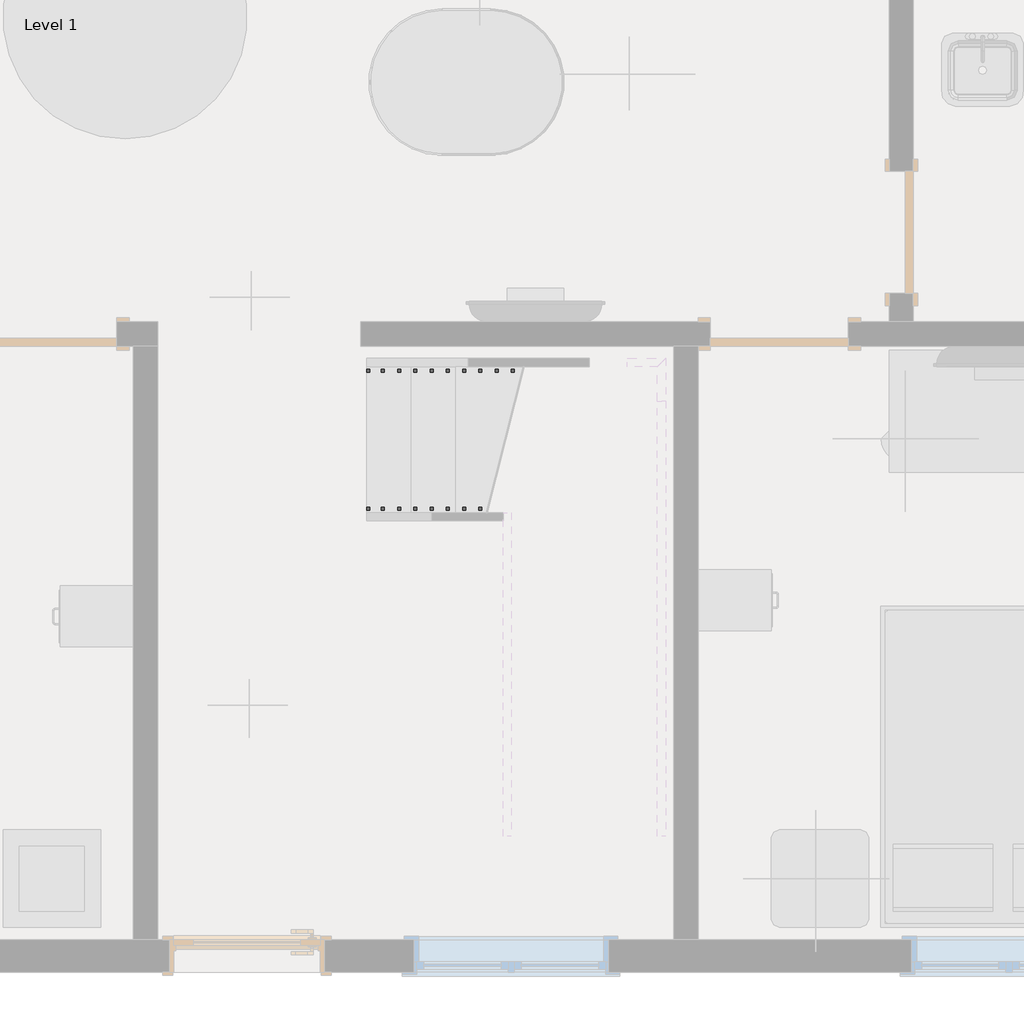
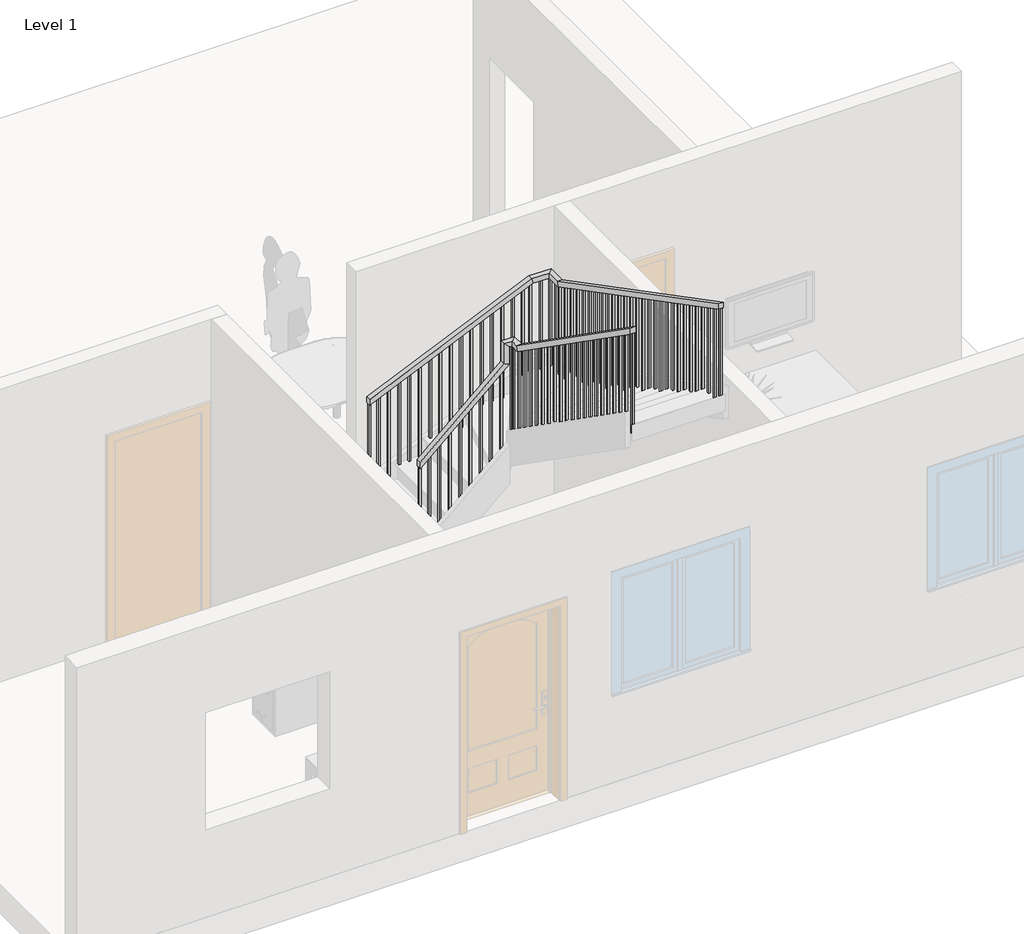
# One storey, part 2 of 3: 2 railings.
"""IFC4 building model written with IfcOpenShell, lengths in millimetres."""

from ifc_helpers import new_model, si_unit, frame, origin, place, context, project, spatial, polyline, outline, extrude, faceted_brep, element, save

model = new_model("IFC4")

# Units and contexts
model_context = context("Model", 3, world=origin())
ifc_project = project(units=[si_unit("LENGTHUNIT", "METRE", prefix="MILLI")], contexts=[model_context])

# Site, building, storey
site = spatial("IfcSite", under=ifc_project)
building = spatial("IfcBuilding", under=site)
storey = spatial("IfcBuildingStorey", under=building, Name="Level 1", Elevation=0.0)

# Railings
placement = place(None, origin())
element("IfcRailing", 1, ObjectType="Handrail - Rectangular", at=placement, inside=storey, context=model_context, shape_type="SolidModel", body=[
    faceted_brep([(-12520.2436952, 5155.3187882, 1682.9646102), (-12520.2436952, 5155.3187882, 1615.1075334), (-12520.2436952, 5104.5187882, 1615.1075334), (-12520.2436952, 5104.5187882, 1682.9646102), (-11692.5067057, 5155.3187882, 2416.0047843), (-11641.7067057, 5155.3187882, 2393.1359601), (-11641.7067057, 5104.5187882, 2393.1359601), (-11692.5067057, 5104.5187882, 2416.0047843), (-11692.5067057, 5155.3187882, 2625.457216), (-11641.7067057, 5155.3187882, 2574.657216), (-11641.7067057, 5104.5187882, 2574.657216), (-11692.5067057, 5104.5187882, 2625.457216), (-11565.5067057, 5155.3187882, 2625.457216), (-11565.5067057, 5155.3187882, 2574.657216), (-11616.3067057, 5104.5187882, 2574.657216), (-11616.3067057, 5104.5187882, 2625.457216), (-11565.5067057, 5028.3187882, 2625.457216), (-11565.5067057, 5012.2891523, 2574.657216), (-11616.3067057, 5012.2891523, 2574.657216), (-11616.3067057, 5028.3187882, 2625.457216), (-11565.5067057, 3082.9817987, 3988.8904479), (-11616.3067057, 3082.9817987, 3988.8904479), (-11616.3067057, 3082.9817987, 3926.8557166), (-11565.5067057, 3082.9817987, 3926.8557166)], [[[0, 1, 2, 3]], [[1, 0, 4, 5]], [[2, 1, 5, 6]], [[3, 2, 6, 7]], [[0, 3, 7, 4]], [[5, 4, 8, 9]], [[6, 5, 9, 10]], [[7, 6, 10, 11]], [[4, 7, 11, 8]], [[9, 8, 12, 13]], [[10, 9, 13, 14]], [[11, 10, 14, 15]], [[8, 11, 15, 12]], [[13, 12, 16, 17]], [[14, 13, 17, 18]], [[15, 14, 18, 19]], [[12, 15, 19, 16]], [[20, 21, 22, 23]], [[17, 16, 20, 23]], [[18, 17, 23, 22]], [[19, 18, 22, 21]], [[16, 19, 21, 20]]]),
    extrude(outline(polyline([(3088.3937882, 3923.0626019), (3107.4437882, 3909.7109805), (3107.4437882, 2878.6666667), (3088.3937882, 2878.6666667), (3088.3937882, 3923.0626019)])), frame((-11600.4317057, 0.0, 0.0), z_axis=(1.0, 0.0, 0.0), x_axis=(0.0, 1.0, 0.0)), (0.0, 0.0, 1.0), 19.05),
    extrude(outline(polyline([(3189.9937882, 3851.8539542), (3209.0437882, 3838.5023328), (3209.0437882, 2878.6666667), (3189.9937882, 2878.6666667), (3189.9937882, 3851.8539542)])), frame((-11600.4317057, 0.0, 0.0), z_axis=(1.0, 0.0, 0.0), x_axis=(0.0, 1.0, 0.0)), (0.0, 0.0, 1.0), 19.05),
    extrude(outline(polyline([(3291.5937882, 3780.6453065), (3310.6437882, 3767.2936851), (3310.6437882, 2878.6666667), (3291.5937882, 2878.6666667), (3291.5937882, 3780.6453065)])), frame((-11600.4317057, 0.0, 0.0), z_axis=(1.0, 0.0, 0.0), x_axis=(0.0, 1.0, 0.0)), (0.0, 0.0, 1.0), 19.05),
    extrude(outline(polyline([(3393.1937882, 3709.4366588), (3412.2437882, 3696.0850374), (3412.2437882, 2709.3333333), (3393.1937882, 2709.3333333), (3393.1937882, 3709.4366588)])), frame((-11600.4317057, 0.0, 0.0), z_axis=(1.0, 0.0, 0.0), x_axis=(0.0, 1.0, 0.0)), (0.0, 0.0, 1.0), 19.05),
    extrude(outline(polyline([(3494.7937882, 3638.2280111), (3513.8437882, 3624.8763897), (3513.8437882, 2709.3333333), (3494.7937882, 2709.3333333), (3494.7937882, 3638.2280111)])), frame((-11600.4317057, 0.0, 0.0), z_axis=(1.0, 0.0, 0.0), x_axis=(0.0, 1.0, 0.0)), (0.0, 0.0, 1.0), 19.05),
    extrude(outline(polyline([(3596.3937882, 3567.0193634), (3615.4437882, 3553.667742), (3615.4437882, 2709.3333333), (3596.3937882, 2709.3333333), (3596.3937882, 3567.0193634)])), frame((-11600.4317057, 0.0, 0.0), z_axis=(1.0, 0.0, 0.0), x_axis=(0.0, 1.0, 0.0)), (0.0, 0.0, 1.0), 19.05),
    extrude(outline(polyline([(3697.9937882, 3495.8107157), (3717.0437882, 3482.4590943), (3717.0437882, 2540.0), (3697.9937882, 2540.0), (3697.9937882, 3495.8107157)])), frame((-11600.4317057, 0.0, 0.0), z_axis=(1.0, 0.0, 0.0), x_axis=(0.0, 1.0, 0.0)), (0.0, 0.0, 1.0), 19.05),
    extrude(outline(polyline([(3799.5937882, 3424.602068), (3818.6437882, 3411.2504466), (3818.6437882, 2540.0), (3799.5937882, 2540.0), (3799.5937882, 3424.602068)])), frame((-11600.4317057, 0.0, 0.0), z_axis=(1.0, 0.0, 0.0), x_axis=(0.0, 1.0, 0.0)), (0.0, 0.0, 1.0), 19.05),
    extrude(outline(polyline([(3901.1937882, 3353.3934203), (3920.2437882, 3340.0417989), (3920.2437882, 2370.6666667), (3901.1937882, 2370.6666667), (3901.1937882, 3353.3934203)])), frame((-11600.4317057, 0.0, 0.0), z_axis=(1.0, 0.0, 0.0), x_axis=(0.0, 1.0, 0.0)), (0.0, 0.0, 1.0), 19.05),
    extrude(outline(polyline([(4002.7937882, 3282.1847726), (4021.8437882, 3268.8331511), (4021.8437882, 2370.6666667), (4002.7937882, 2370.6666667), (4002.7937882, 3282.1847726)])), frame((-11600.4317057, 0.0, 0.0), z_axis=(1.0, 0.0, 0.0), x_axis=(0.0, 1.0, 0.0)), (0.0, 0.0, 1.0), 19.05),
    extrude(outline(polyline([(4104.3937882, 3210.9761249), (4123.4437882, 3197.6245034), (4123.4437882, 2370.6666667), (4104.3937882, 2370.6666667), (4104.3937882, 3210.9761249)])), frame((-11600.4317057, 0.0, 0.0), z_axis=(1.0, 0.0, 0.0), x_axis=(0.0, 1.0, 0.0)), (0.0, 0.0, 1.0), 19.05),
    extrude(outline(polyline([(4205.9937882, 3139.7674772), (4225.0437882, 3126.4158557), (4225.0437882, 2201.3333333), (4205.9937882, 2201.3333333), (4205.9937882, 3139.7674772)])), frame((-11600.4317057, 0.0, 0.0), z_axis=(1.0, 0.0, 0.0), x_axis=(0.0, 1.0, 0.0)), (0.0, 0.0, 1.0), 19.05),
    extrude(outline(polyline([(4307.5937882, 3068.5588295), (4326.6437882, 3055.207208), (4326.6437882, 2201.3333333), (4307.5937882, 2201.3333333), (4307.5937882, 3068.5588295)])), frame((-11600.4317057, 0.0, 0.0), z_axis=(1.0, 0.0, 0.0), x_axis=(0.0, 1.0, 0.0)), (0.0, 0.0, 1.0), 19.05),
    extrude(outline(polyline([(4409.1937882, 2997.3501818), (4428.2437882, 2983.9985603), (4428.2437882, 2201.3333333), (4409.1937882, 2201.3333333), (4409.1937882, 2997.3501818)])), frame((-11600.4317057, 0.0, 0.0), z_axis=(1.0, 0.0, 0.0), x_axis=(0.0, 1.0, 0.0)), (0.0, 0.0, 1.0), 19.05),
    extrude(outline(polyline([(4510.7937882, 2926.1415341), (4529.8437882, 2912.7899126), (4529.8437882, 2032.0), (4510.7937882, 2032.0), (4510.7937882, 2926.1415341)])), frame((-11600.4317057, 0.0, 0.0), z_axis=(1.0, 0.0, 0.0), x_axis=(0.0, 1.0, 0.0)), (0.0, 0.0, 1.0), 19.05),
    extrude(outline(polyline([(4612.3937882, 2854.9328864), (4631.4437882, 2841.5812649), (4631.4437882, 2032.0), (4612.3937882, 2032.0), (4612.3937882, 2854.9328864)])), frame((-11600.4317057, 0.0, 0.0), z_axis=(1.0, 0.0, 0.0), x_axis=(0.0, 1.0, 0.0)), (0.0, 0.0, 1.0), 19.05),
    extrude(outline(polyline([(4713.9937882, 2783.7242387), (4733.0437882, 2770.3726172), (4733.0437882, 1862.6666667), (4713.9937882, 1862.6666667), (4713.9937882, 2783.7242387)])), frame((-11600.4317057, 0.0, 0.0), z_axis=(1.0, 0.0, 0.0), x_axis=(0.0, 1.0, 0.0)), (0.0, 0.0, 1.0), 19.05),
    extrude(outline(polyline([(4815.5937882, 2712.515591), (4834.6437882, 2699.1639695), (4834.6437882, 1862.6666667), (4815.5937882, 1862.6666667), (4815.5937882, 2712.515591)])), frame((-11600.4317057, 0.0, 0.0), z_axis=(1.0, 0.0, 0.0), x_axis=(0.0, 1.0, 0.0)), (0.0, 0.0, 1.0), 19.05),
    extrude(outline(polyline([(4917.1937882, 2641.3069432), (4936.2437882, 2627.9553218), (4936.2437882, 1693.3333333), (4917.1937882, 1693.3333333), (4917.1937882, 2641.3069432)])), frame((-11600.4317057, 0.0, 0.0), z_axis=(1.0, 0.0, 0.0), x_axis=(0.0, 1.0, 0.0)), (0.0, 0.0, 1.0), 19.05),
    extrude(outline(polyline([(-11600.4317057, 5037.8437882), (-11581.3817057, 5037.8437882), (-11581.3817057, 5018.7937882), (-11600.4317057, 5018.7937882), (-11600.4317057, 5037.8437882)])), frame((0.0, 0.0, 1693.3333333), z_axis=(0.0, 0.0, 1.0), x_axis=(1.0, 0.0, 0.0)), (0.0, 0.0, 1.0), 881.3238827),
    extrude(outline(polyline([(-11615.3686952, 5120.3937882), (-11615.3686952, 5139.4437882), (-11596.3186952, 5139.4437882), (-11596.3186952, 5120.3937882), (-11615.3686952, 5120.3937882)])), frame((0.0, 0.0, 1524.0), z_axis=(0.0, 0.0, 1.0), x_axis=(1.0, 0.0, 0.0)), (0.0, 0.0, 1.0), 1050.657216),
    extrude(outline(polyline([(2343.3548737, -11697.9186952), (2326.484279, -11716.9686952), (1354.6666667, -11716.9686952), (1354.6666667, -11697.9186952), (2343.3548737, -11697.9186952)])), frame((0.0, 5120.3937882, 0.0), z_axis=(0.0, 1.0, 0.0), x_axis=(0.0, 0.0, 1.0)), (0.0, 0.0, 1.0), 19.05),
    extrude(outline(polyline([(2253.3783684, -11799.5186952), (2236.5077736, -11818.5686952), (1185.3333333, -11818.5686952), (1185.3333333, -11799.5186952), (2253.3783684, -11799.5186952)])), frame((0.0, 5120.3937882, 0.0), z_axis=(0.0, 1.0, 0.0), x_axis=(0.0, 0.0, 1.0)), (0.0, 0.0, 1.0), 19.05),
    extrude(outline(polyline([(2163.401863, -11901.1186952), (2146.5312682, -11920.1686952), (1185.3333333, -11920.1686952), (1185.3333333, -11901.1186952), (2163.401863, -11901.1186952)])), frame((0.0, 5120.3937882, 0.0), z_axis=(0.0, 1.0, 0.0), x_axis=(0.0, 0.0, 1.0)), (0.0, 0.0, 1.0), 19.05),
    extrude(outline(polyline([(2073.4253576, -12002.7186952), (2056.5547629, -12021.7686952), (1016.0, -12021.7686952), (1016.0, -12002.7186952), (2073.4253576, -12002.7186952)])), frame((0.0, 5120.3937882, 0.0), z_axis=(0.0, 1.0, 0.0), x_axis=(0.0, 0.0, 1.0)), (0.0, 0.0, 1.0), 19.05),
    extrude(outline(polyline([(1983.4488522, -12104.3186952), (1966.5782575, -12123.3686952), (1016.0, -12123.3686952), (1016.0, -12104.3186952), (1983.4488522, -12104.3186952)])), frame((0.0, 5120.3937882, 0.0), z_axis=(0.0, 1.0, 0.0), x_axis=(0.0, 0.0, 1.0)), (0.0, 0.0, 1.0), 19.05),
    extrude(outline(polyline([(1893.4723469, -12205.9186952), (1876.6017521, -12224.9686952), (1016.0, -12224.9686952), (1016.0, -12205.9186952), (1893.4723469, -12205.9186952)])), frame((0.0, 5120.3937882, 0.0), z_axis=(0.0, 1.0, 0.0), x_axis=(0.0, 0.0, 1.0)), (0.0, 0.0, 1.0), 19.05),
    extrude(outline(polyline([(1803.4958415, -12307.5186952), (1786.6252467, -12326.5686952), (846.6666667, -12326.5686952), (846.6666667, -12307.5186952), (1803.4958415, -12307.5186952)])), frame((0.0, 5120.3937882, 0.0), z_axis=(0.0, 1.0, 0.0), x_axis=(0.0, 0.0, 1.0)), (0.0, 0.0, 1.0), 19.05),
    extrude(outline(polyline([(1713.5193361, -12409.1186952), (1696.6487414, -12428.1686952), (846.6666667, -12428.1686952), (846.6666667, -12409.1186952), (1713.5193361, -12409.1186952)])), frame((0.0, 5120.3937882, 0.0), z_axis=(0.0, 1.0, 0.0), x_axis=(0.0, 0.0, 1.0)), (0.0, 0.0, 1.0), 19.05),
    extrude(outline(polyline([(-11600.4317057, 5139.4437882), (-11581.3817057, 5139.4437882), (-11581.3817057, 5120.3937882), (-11600.4317057, 5120.3937882), (-11600.4317057, 5139.4437882)])), frame((0.0, 0.0, 1524.0), z_axis=(0.0, 0.0, 1.0), x_axis=(1.0, 0.0, 0.0)), (0.0, 0.0, 1.0), 1050.657216),
    extrude(outline(polyline([(3082.9817987, 3926.8557166), (3102.0317987, 3913.5040952), (3102.0317987, 2878.6666667), (3082.9817987, 2878.6666667), (3082.9817987, 3926.8557166)])), frame((-11600.4317057, 0.0, 0.0), z_axis=(1.0, 0.0, 0.0), x_axis=(0.0, 1.0, 0.0)), (0.0, 0.0, 1.0), 19.05),
    extrude(outline(polyline([(1631.9781281, -12501.1936952), (1615.1075334, -12520.2436952), (846.6666667, -12520.2436952), (846.6666667, -12501.1936952), (1631.9781281, -12501.1936952)])), frame((0.0, 5120.3937882, 0.0), z_axis=(0.0, 1.0, 0.0), x_axis=(0.0, 0.0, 1.0)), (0.0, 0.0, 1.0), 19.05),
])
element("IfcRailing", 2, ObjectType="Handrail - Rectangular", at=placement, inside=storey, context=model_context, shape_type="SolidModel", body=[
    faceted_brep([(-12520.2436952, 6018.9187882, 1807.8545254), (-12520.2436952, 6018.9187882, 1752.3830665), (-12520.2436952, 5968.1187882, 1752.3830665), (-12520.2436952, 5968.1187882, 1807.8545254), (-10922.8906609, 6018.9187882, 2508.4571941), (-10912.2398749, 6018.9187882, 2457.6571941), (-10912.2398749, 5968.1187882, 2457.6571941), (-10922.8906609, 5968.1187882, 2508.4571941), (-10701.9067057, 6018.9187882, 2508.4571941), (-10701.9067057, 6018.9187882, 2457.6571941), (-10752.7067057, 5968.1187882, 2457.6571941), (-10752.7067057, 5968.1187882, 2508.4571941), (-10701.9067057, 5828.8154443, 2508.4571941), (-10701.9067057, 5816.3790497, 2457.6571941), (-10752.7067057, 5816.3790497, 2457.6571941), (-10752.7067057, 5828.8154443, 2508.4571941), (-10701.9067057, 3082.9817987, 3938.588476), (-10752.7067057, 3082.9817987, 3938.588476), (-10752.7067057, 3082.9817987, 3881.3111437), (-10701.9067057, 3082.9817987, 3881.3111437)], [[[0, 1, 2, 3]], [[1, 0, 4, 5]], [[2, 1, 5, 6]], [[3, 2, 6, 7]], [[0, 3, 7, 4]], [[5, 4, 8, 9]], [[6, 5, 9, 10]], [[7, 6, 10, 11]], [[4, 7, 11, 8]], [[9, 8, 12, 13]], [[10, 9, 13, 14]], [[11, 10, 14, 15]], [[8, 11, 15, 12]], [[16, 17, 18, 19]], [[13, 12, 16, 19]], [[14, 13, 19, 18]], [[15, 14, 18, 17]], [[12, 15, 17, 16]]]),
    extrude(outline(polyline([(3095.1404443, 3874.9727949), (3095.1404443, 2878.6666667), (3076.0904443, 2878.6666667), (3076.0904443, 3884.8947365), (3095.1404443, 3874.9727949)])), frame((-10736.8317057, 0.0, 0.0), z_axis=(1.0, 0.0, 0.0), x_axis=(0.0, 1.0, 0.0)), (0.0, 0.0, 1.0), 19.05),
    extrude(outline(polyline([(3196.7404443, 3822.0557734), (3196.7404443, 2878.6666667), (3177.6904443, 2878.6666667), (3177.6904443, 3831.9777149), (3196.7404443, 3822.0557734)])), frame((-10736.8317057, 0.0, 0.0), z_axis=(1.0, 0.0, 0.0), x_axis=(0.0, 1.0, 0.0)), (0.0, 0.0, 1.0), 19.05),
    extrude(outline(polyline([(3298.3404443, 3769.1444302), (3298.3404443, 2878.6666667), (3279.2904443, 2878.6666667), (3279.2904443, 3779.0663717), (3298.3404443, 3769.1444302)])), frame((-10736.8317057, 0.0, 0.0), z_axis=(1.0, 0.0, 0.0), x_axis=(0.0, 1.0, 0.0)), (0.0, 0.0, 1.0), 19.05),
    extrude(outline(polyline([(3399.9404443, 3716.2217303), (3399.9404443, 2709.3333333), (3380.8904443, 2709.3333333), (3380.8904443, 3726.1436718), (3399.9404443, 3716.2217303)])), frame((-10736.8317057, 0.0, 0.0), z_axis=(1.0, 0.0, 0.0), x_axis=(0.0, 1.0, 0.0)), (0.0, 0.0, 1.0), 19.05),
    extrude(outline(polyline([(3501.5404443, 3663.3047087), (3501.5404443, 2709.3333333), (3482.4904443, 2709.3333333), (3482.4904443, 3673.2266502), (3501.5404443, 3663.3047087)])), frame((-10736.8317057, 0.0, 0.0), z_axis=(1.0, 0.0, 0.0), x_axis=(0.0, 1.0, 0.0)), (0.0, 0.0, 1.0), 19.05),
    extrude(outline(polyline([(3603.1404443, 3610.3933655), (3603.1404443, 2709.3333333), (3584.0904443, 2709.3333333), (3584.0904443, 3620.315307), (3603.1404443, 3610.3933655)])), frame((-10736.8317057, 0.0, 0.0), z_axis=(1.0, 0.0, 0.0), x_axis=(0.0, 1.0, 0.0)), (0.0, 0.0, 1.0), 19.05),
    extrude(outline(polyline([(3704.7404443, 3557.4706656), (3704.7404443, 2540.0), (3685.6904443, 2540.0), (3685.6904443, 3567.3926071), (3704.7404443, 3557.4706656)])), frame((-10736.8317057, 0.0, 0.0), z_axis=(1.0, 0.0, 0.0), x_axis=(0.0, 1.0, 0.0)), (0.0, 0.0, 1.0), 19.05),
    extrude(outline(polyline([(3806.3404443, 3504.553644), (3806.3404443, 2540.0), (3787.2904443, 2540.0), (3787.2904443, 3514.4755855), (3806.3404443, 3504.553644)])), frame((-10736.8317057, 0.0, 0.0), z_axis=(1.0, 0.0, 0.0), x_axis=(0.0, 1.0, 0.0)), (0.0, 0.0, 1.0), 19.05),
    extrude(outline(polyline([(3907.9404443, 3451.6366224), (3907.9404443, 2540.0), (3888.8904443, 2540.0), (3888.8904443, 3461.558564), (3907.9404443, 3451.6366224)])), frame((-10736.8317057, 0.0, 0.0), z_axis=(1.0, 0.0, 0.0), x_axis=(0.0, 1.0, 0.0)), (0.0, 0.0, 1.0), 19.05),
    extrude(outline(polyline([(4009.5404443, 3398.7196009), (4009.5404443, 2370.6666667), (3990.4904443, 2370.6666667), (3990.4904443, 3408.6415424), (4009.5404443, 3398.7196009)])), frame((-10736.8317057, 0.0, 0.0), z_axis=(1.0, 0.0, 0.0), x_axis=(0.0, 1.0, 0.0)), (0.0, 0.0, 1.0), 19.05),
    extrude(outline(polyline([(4111.1404443, 3345.8025793), (4111.1404443, 2370.6666667), (4092.0904443, 2370.6666667), (4092.0904443, 3355.7245208), (4111.1404443, 3345.8025793)])), frame((-10736.8317057, 0.0, 0.0), z_axis=(1.0, 0.0, 0.0), x_axis=(0.0, 1.0, 0.0)), (0.0, 0.0, 1.0), 19.05),
    extrude(outline(polyline([(4212.7404443, 3292.8912361), (4212.7404443, 2370.6666667), (4193.6904443, 2370.6666667), (4193.6904443, 3302.8131776), (4212.7404443, 3292.8912361)])), frame((-10736.8317057, 0.0, 0.0), z_axis=(1.0, 0.0, 0.0), x_axis=(0.0, 1.0, 0.0)), (0.0, 0.0, 1.0), 19.05),
    extrude(outline(polyline([(4314.3404443, 3239.9742145), (4314.3404443, 2201.3333333), (4295.2904443, 2201.3333333), (4295.2904443, 3249.8961561), (4314.3404443, 3239.9742145)])), frame((-10736.8317057, 0.0, 0.0), z_axis=(1.0, 0.0, 0.0), x_axis=(0.0, 1.0, 0.0)), (0.0, 0.0, 1.0), 19.05),
    extrude(outline(polyline([(4415.9404443, 3187.057193), (4415.9404443, 2201.3333333), (4396.8904443, 2201.3333333), (4396.8904443, 3196.9791345), (4415.9404443, 3187.057193)])), frame((-10736.8317057, 0.0, 0.0), z_axis=(1.0, 0.0, 0.0), x_axis=(0.0, 1.0, 0.0)), (0.0, 0.0, 1.0), 19.05),
    extrude(outline(polyline([(4517.5404443, 3134.1401714), (4517.5404443, 2201.3333333), (4498.4904443, 2201.3333333), (4498.4904443, 3144.062113), (4517.5404443, 3134.1401714)])), frame((-10736.8317057, 0.0, 0.0), z_axis=(1.0, 0.0, 0.0), x_axis=(0.0, 1.0, 0.0)), (0.0, 0.0, 1.0), 19.05),
    extrude(outline(polyline([(4619.1404443, 3081.2231498), (4619.1404443, 2032.0), (4600.0904443, 2032.0), (4600.0904443, 3091.1450914), (4619.1404443, 3081.2231498)])), frame((-10736.8317057, 0.0, 0.0), z_axis=(1.0, 0.0, 0.0), x_axis=(0.0, 1.0, 0.0)), (0.0, 0.0, 1.0), 19.05),
    extrude(outline(polyline([(4720.7404443, 3028.3061283), (4720.7404443, 2032.0), (4701.6904443, 2032.0), (4701.6904443, 3038.2280698), (4720.7404443, 3028.3061283)])), frame((-10736.8317057, 0.0, 0.0), z_axis=(1.0, 0.0, 0.0), x_axis=(0.0, 1.0, 0.0)), (0.0, 0.0, 1.0), 19.05),
    extrude(outline(polyline([(4822.3404443, 2975.3891067), (4822.3404443, 2032.0), (4803.2904443, 2032.0), (4803.2904443, 2985.3110483), (4822.3404443, 2975.3891067)])), frame((-10736.8317057, 0.0, 0.0), z_axis=(1.0, 0.0, 0.0), x_axis=(0.0, 1.0, 0.0)), (0.0, 0.0, 1.0), 19.05),
    extrude(outline(polyline([(4923.9404443, 2922.4720852), (4923.9404443, 1862.6666667), (4904.8904443, 1862.6666667), (4904.8904443, 2932.3940267), (4923.9404443, 2922.4720852)])), frame((-10736.8317057, 0.0, 0.0), z_axis=(1.0, 0.0, 0.0), x_axis=(0.0, 1.0, 0.0)), (0.0, 0.0, 1.0), 19.05),
    extrude(outline(polyline([(5025.5404443, 2869.5550636), (5025.5404443, 1862.6666667), (5006.4904443, 1862.6666667), (5006.4904443, 2879.4770051), (5025.5404443, 2869.5550636)])), frame((-10736.8317057, 0.0, 0.0), z_axis=(1.0, 0.0, 0.0), x_axis=(0.0, 1.0, 0.0)), (0.0, 0.0, 1.0), 19.05),
    extrude(outline(polyline([(5127.1404443, 2816.638042), (5127.1404443, 1862.6666667), (5108.0904443, 1862.6666667), (5108.0904443, 2826.5599836), (5127.1404443, 2816.638042)])), frame((-10736.8317057, 0.0, 0.0), z_axis=(1.0, 0.0, 0.0), x_axis=(0.0, 1.0, 0.0)), (0.0, 0.0, 1.0), 19.05),
    extrude(outline(polyline([(5228.7404443, 2763.7210205), (5228.7404443, 1693.3333333), (5209.6904443, 1693.3333333), (5209.6904443, 2773.642962), (5228.7404443, 2763.7210205)])), frame((-10736.8317057, 0.0, 0.0), z_axis=(1.0, 0.0, 0.0), x_axis=(0.0, 1.0, 0.0)), (0.0, 0.0, 1.0), 19.05),
    extrude(outline(polyline([(5330.3404443, 2710.8039989), (5330.3404443, 1693.3333333), (5311.2904443, 1693.3333333), (5311.2904443, 2720.7259404), (5330.3404443, 2710.8039989)])), frame((-10736.8317057, 0.0, 0.0), z_axis=(1.0, 0.0, 0.0), x_axis=(0.0, 1.0, 0.0)), (0.0, 0.0, 1.0), 19.05),
    extrude(outline(polyline([(5431.9404443, 2657.8869773), (5431.9404443, 1693.3333333), (5412.8904443, 1693.3333333), (5412.8904443, 2667.8089189), (5431.9404443, 2657.8869773)])), frame((-10736.8317057, 0.0, 0.0), z_axis=(1.0, 0.0, 0.0), x_axis=(0.0, 1.0, 0.0)), (0.0, 0.0, 1.0), 19.05),
    extrude(outline(polyline([(5533.5404443, 2604.9699558), (5533.5404443, 1693.3333333), (5514.4904443, 1693.3333333), (5514.4904443, 2614.8918973), (5533.5404443, 2604.9699558)])), frame((-10736.8317057, 0.0, 0.0), z_axis=(1.0, 0.0, 0.0), x_axis=(0.0, 1.0, 0.0)), (0.0, 0.0, 1.0), 19.05),
    extrude(outline(polyline([(5635.1404443, 2552.0529342), (5635.1404443, 1524.0), (5616.0904443, 1524.0), (5616.0904443, 2561.9748757), (5635.1404443, 2552.0529342)])), frame((-10736.8317057, 0.0, 0.0), z_axis=(1.0, 0.0, 0.0), x_axis=(0.0, 1.0, 0.0)), (0.0, 0.0, 1.0), 19.05),
    extrude(outline(polyline([(5736.7404443, 2499.1359126), (5736.7404443, 1524.0), (5717.6904443, 1524.0), (5717.6904443, 2509.0578542), (5736.7404443, 2499.1359126)])), frame((-10736.8317057, 0.0, 0.0), z_axis=(1.0, 0.0, 0.0), x_axis=(0.0, 1.0, 0.0)), (0.0, 0.0, 1.0), 19.05),
    extrude(outline(polyline([(-10717.7817057, 5901.4437882), (-10717.7817057, 5882.3937882), (-10736.8317057, 5882.3937882), (-10736.8317057, 5901.4437882), (-10717.7817057, 5901.4437882)])), frame((0.0, 0.0, 1524.0), z_axis=(0.0, 0.0, 1.0), x_axis=(1.0, 0.0, 0.0)), (0.0, 0.0, 1.0), 933.6571941),
    extrude(outline(polyline([(-10830.8156609, 6003.0437882), (-10811.7656609, 6003.0437882), (-10811.7656609, 5983.9937882), (-10830.8156609, 5983.9937882), (-10830.8156609, 6003.0437882)])), frame((0.0, 0.0, 1524.0), z_axis=(0.0, 0.0, 1.0), x_axis=(1.0, 0.0, 0.0)), (0.0, 0.0, 1.0), 933.6571941),
    extrude(outline(polyline([(2416.6352411, -11005.7686952), (1524.0, -11005.7686952), (1524.0, -10986.7186952), (2424.9906144, -10986.7186952), (2416.6352411, -11005.7686952)])), frame((0.0, 5983.9937882, 0.0), z_axis=(0.0, 1.0, 0.0), x_axis=(0.0, 0.0, 1.0)), (0.0, 0.0, 1.0), 19.05),
    extrude(outline(polyline([(2372.0732504, -11107.3686952), (1524.0, -11107.3686952), (1524.0, -11088.3186952), (2380.4286236, -11088.3186952), (2372.0732504, -11107.3686952)])), frame((0.0, 5983.9937882, 0.0), z_axis=(0.0, 1.0, 0.0), x_axis=(0.0, 0.0, 1.0)), (0.0, 0.0, 1.0), 19.05),
    extrude(outline(polyline([(2327.5112596, -11208.9686952), (1354.6666667, -11208.9686952), (1354.6666667, -11189.9186952), (2335.8666329, -11189.9186952), (2327.5112596, -11208.9686952)])), frame((0.0, 5983.9937882, 0.0), z_axis=(0.0, 1.0, 0.0), x_axis=(0.0, 0.0, 1.0)), (0.0, 0.0, 1.0), 19.05),
    extrude(outline(polyline([(2282.9492689, -11310.5686952), (1354.6666667, -11310.5686952), (1354.6666667, -11291.5186952), (2291.3046421, -11291.5186952), (2282.9492689, -11310.5686952)])), frame((0.0, 5983.9937882, 0.0), z_axis=(0.0, 1.0, 0.0), x_axis=(0.0, 0.0, 1.0)), (0.0, 0.0, 1.0), 19.05),
    extrude(outline(polyline([(2238.3872781, -11412.1686952), (1354.6666667, -11412.1686952), (1354.6666667, -11393.1186952), (2246.7426514, -11393.1186952), (2238.3872781, -11412.1686952)])), frame((0.0, 5983.9937882, 0.0), z_axis=(0.0, 1.0, 0.0), x_axis=(0.0, 0.0, 1.0)), (0.0, 0.0, 1.0), 19.05),
    extrude(outline(polyline([(2193.8252874, -11513.7686952), (1354.6666667, -11513.7686952), (1354.6666667, -11494.7186952), (2202.1806606, -11494.7186952), (2193.8252874, -11513.7686952)])), frame((0.0, 5983.9937882, 0.0), z_axis=(0.0, 1.0, 0.0), x_axis=(0.0, 0.0, 1.0)), (0.0, 0.0, 1.0), 19.05),
    extrude(outline(polyline([(2149.2632966, -11615.3686952), (1185.3333333, -11615.3686952), (1185.3333333, -11596.3186952), (2157.6186699, -11596.3186952), (2149.2632966, -11615.3686952)])), frame((0.0, 5983.9937882, 0.0), z_axis=(0.0, 1.0, 0.0), x_axis=(0.0, 0.0, 1.0)), (0.0, 0.0, 1.0), 19.05),
    extrude(outline(polyline([(2104.7013059, -11716.9686952), (1185.3333333, -11716.9686952), (1185.3333333, -11697.9186952), (2113.0566791, -11697.9186952), (2104.7013059, -11716.9686952)])), frame((0.0, 5983.9937882, 0.0), z_axis=(0.0, 1.0, 0.0), x_axis=(0.0, 0.0, 1.0)), (0.0, 0.0, 1.0), 19.05),
    extrude(outline(polyline([(2060.1393151, -11818.5686952), (1185.3333333, -11818.5686952), (1185.3333333, -11799.5186952), (2068.4946884, -11799.5186952), (2060.1393151, -11818.5686952)])), frame((0.0, 5983.9937882, 0.0), z_axis=(0.0, 1.0, 0.0), x_axis=(0.0, 0.0, 1.0)), (0.0, 0.0, 1.0), 19.05),
    extrude(outline(polyline([(2015.5773244, -11920.1686952), (1185.3333333, -11920.1686952), (1185.3333333, -11901.1186952), (2023.9326976, -11901.1186952), (2015.5773244, -11920.1686952)])), frame((0.0, 5983.9937882, 0.0), z_axis=(0.0, 1.0, 0.0), x_axis=(0.0, 0.0, 1.0)), (0.0, 0.0, 1.0), 19.05),
    extrude(outline(polyline([(1971.0153336, -12021.7686952), (1016.0, -12021.7686952), (1016.0, -12002.7186952), (1979.3707069, -12002.7186952), (1971.0153336, -12021.7686952)])), frame((0.0, 5983.9937882, 0.0), z_axis=(0.0, 1.0, 0.0), x_axis=(0.0, 0.0, 1.0)), (0.0, 0.0, 1.0), 19.05),
    extrude(outline(polyline([(1926.4533429, -12123.3686952), (1016.0, -12123.3686952), (1016.0, -12104.3186952), (1934.8087161, -12104.3186952), (1926.4533429, -12123.3686952)])), frame((0.0, 5983.9937882, 0.0), z_axis=(0.0, 1.0, 0.0), x_axis=(0.0, 0.0, 1.0)), (0.0, 0.0, 1.0), 19.05),
    extrude(outline(polyline([(1881.8913521, -12224.9686952), (1016.0, -12224.9686952), (1016.0, -12205.9186952), (1890.2467254, -12205.9186952), (1881.8913521, -12224.9686952)])), frame((0.0, 5983.9937882, 0.0), z_axis=(0.0, 1.0, 0.0), x_axis=(0.0, 0.0, 1.0)), (0.0, 0.0, 1.0), 19.05),
    extrude(outline(polyline([(1837.3293614, -12326.5686952), (846.6666667, -12326.5686952), (846.6666667, -12307.5186952), (1845.6847346, -12307.5186952), (1837.3293614, -12326.5686952)])), frame((0.0, 5983.9937882, 0.0), z_axis=(0.0, 1.0, 0.0), x_axis=(0.0, 0.0, 1.0)), (0.0, 0.0, 1.0), 19.05),
    extrude(outline(polyline([(1792.7673706, -12428.1686952), (846.6666667, -12428.1686952), (846.6666667, -12409.1186952), (1801.1227439, -12409.1186952), (1792.7673706, -12428.1686952)])), frame((0.0, 5983.9937882, 0.0), z_axis=(0.0, 1.0, 0.0), x_axis=(0.0, 0.0, 1.0)), (0.0, 0.0, 1.0), 19.05),
    extrude(outline(polyline([(-10717.7817057, 5838.3404443), (-10717.7817057, 5819.2904443), (-10736.8317057, 5819.2904443), (-10736.8317057, 5838.3404443), (-10717.7817057, 5838.3404443)])), frame((0.0, 0.0, 1524.0), z_axis=(0.0, 0.0, 1.0), x_axis=(1.0, 0.0, 0.0)), (0.0, 0.0, 1.0), 933.6571941),
    extrude(outline(polyline([(-10736.8317057, 6003.0437882), (-10717.7817057, 6003.0437882), (-10717.7817057, 5983.9937882), (-10736.8317057, 5983.9937882), (-10736.8317057, 6003.0437882)])), frame((0.0, 0.0, 1524.0), z_axis=(0.0, 0.0, 1.0), x_axis=(1.0, 0.0, 0.0)), (0.0, 0.0, 1.0), 933.6571941),
    extrude(outline(polyline([(2448.8080486, -10932.4156609), (1524.0, -10932.4156609), (1524.0, -10913.3656609), (2457.1634218, -10913.3656609), (2448.8080486, -10932.4156609)])), frame((0.0, 5983.9937882, 0.0), z_axis=(0.0, 1.0, 0.0), x_axis=(0.0, 0.0, 1.0)), (0.0, 0.0, 1.0), 19.05),
    extrude(outline(polyline([(3102.0317987, 3871.3892021), (3102.0317987, 2878.6666667), (3082.9817987, 2878.6666667), (3082.9817987, 3881.3111437), (3102.0317987, 3871.3892021)])), frame((-10736.8317057, 0.0, 0.0), z_axis=(1.0, 0.0, 0.0), x_axis=(0.0, 1.0, 0.0)), (0.0, 0.0, 1.0), 19.05),
    extrude(outline(polyline([(1752.3830665, -12520.2436952), (846.6666667, -12520.2436952), (846.6666667, -12501.1936952), (1760.7384398, -12501.1936952), (1752.3830665, -12520.2436952)])), frame((0.0, 5983.9937882, 0.0), z_axis=(0.0, 1.0, 0.0), x_axis=(0.0, 0.0, 1.0)), (0.0, 0.0, 1.0), 19.05),
])

save(model, "model.ifc")

# Revit data of these elements
# Type "Handrail - Rectangular"
#   Assembly Code = "C2010400"
#   built-in parameter 1008612 = 0.0416667 (stored number, unit not read)
#   built-in parameter 1008611 = 0.0416667 (stored number, unit not read)
#   built-in parameter 1008609 = 0.333333 (stored number, unit not read)
#   built-in parameter 1008604 = 0.166667 (stored number, unit not read)
#   built-in parameter 1008603 = 0.166667 (stored number, unit not read)
#   Railing Height = 3' - 0"
#   built-in parameter 1008630 = 2
#   built-in parameter 1008610 = 2
#   built-in parameter 1008618 = Baluster - Square : 3/4"
# Elements 1, 2 (IfcRailing, "Handrail - Rectangular")
#   Phase Created = New Construction
